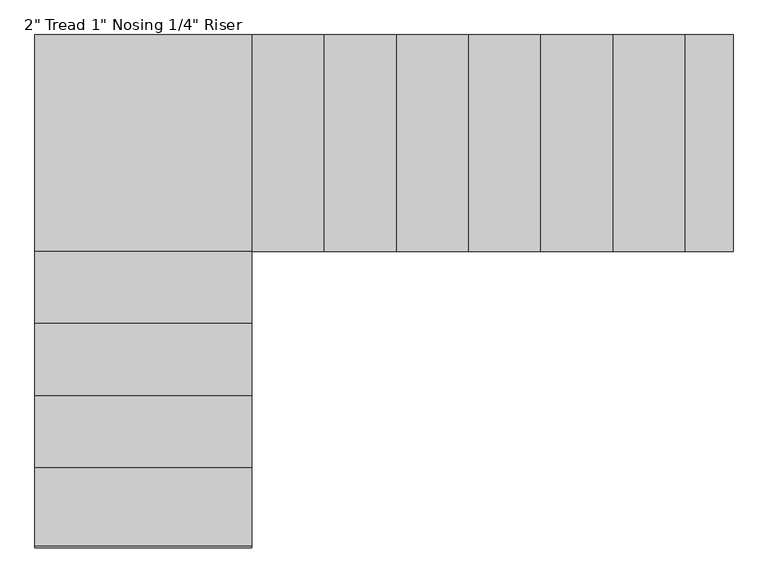
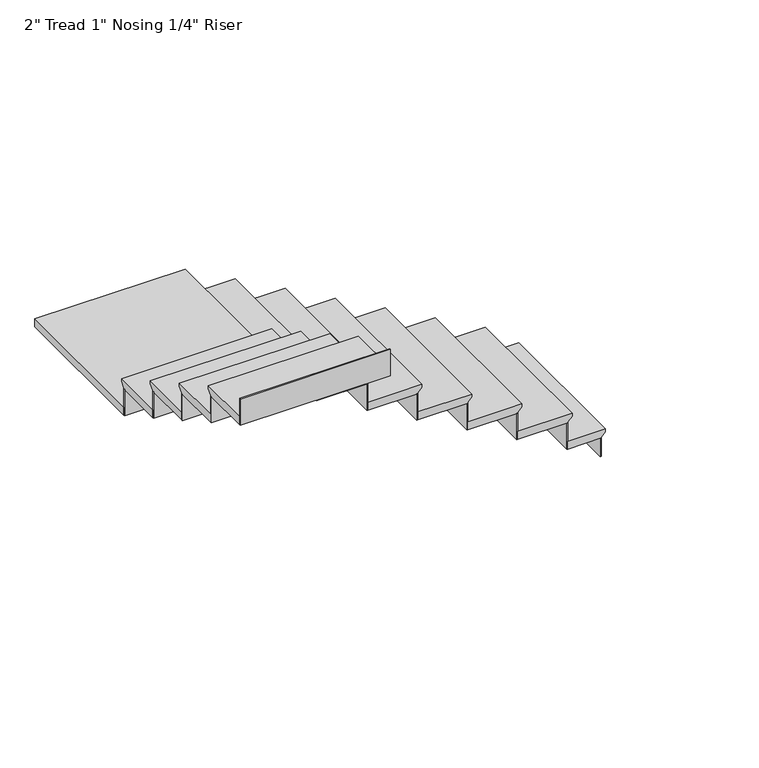
"""IFC4 building model written with IfcOpenShell, lengths in millimetres: stair flight geometry."""

from ifc_helpers import new_model, si_unit, origin, place, context, project, spatial, faceted_brep, source, transform, mapped, element, save


def stair_flight_aa7d7887(model_context):
    return source(origin(), model_context, "Body", "Brep", [
        faceted_brep([(-442.4415084, 5282.3381995, 9599.0833333), (-442.4415084, 5282.3381995, 9618.1333333), (-442.4415084, 4368.3146777, 9618.1333333), (-442.4415084, 4368.3146777, 9599.0833333), (-467.8415084, 5282.3381995, 9573.6833333), (-467.8415084, 4368.3146777, 9573.6833333), (-671.0415084, 5282.3381995, 9618.1333333), (-671.0415084, 4368.3146777, 9618.1333333), (-467.8415084, 4368.3146777, 9567.3333333), (-671.0415084, 4368.3146777, 9567.3333333), (-671.0415084, 5282.3381995, 9567.3333333), (-467.8415084, 5282.3381995, 9567.3333333)], [[[0, 1, 2, 3]], [[4, 0, 3, 5]], [[2, 1, 6, 7]], [[8, 9, 10, 11]], [[2, 7, 9, 8, 5, 3]], [[8, 11, 4, 5]], [[6, 1, 0, 4, 11, 10]], [[7, 6, 10, 9]]]),
        faceted_brep([(-467.8415084, 5282.3381995, 9567.3333333), (-467.8415084, 5282.3381995, 9448.8), (-474.1915084, 5282.3381995, 9448.8), (-474.1915084, 5282.3381995, 9567.3333333), (-467.8415084, 4368.3146777, 9567.3333333), (-474.1915084, 4368.3146777, 9567.3333333), (-474.1915084, 4368.3146777, 9448.8), (-467.8415084, 4368.3146777, 9448.8)], [[[0, 1, 2, 3]], [[4, 5, 6, 7]], [[1, 0, 4, 7]], [[2, 1, 7, 6]], [[3, 2, 6, 5]], [[0, 3, 5, 4]]]),
        faceted_brep([(-671.0415084, 5282.3381995, 9736.6666667), (-671.0415084, 5282.3381995, 9567.3333333), (-677.3915084, 5282.3381995, 9567.3333333), (-677.3915084, 5282.3381995, 9736.6666667), (-671.0415084, 4368.3146777, 9736.6666667), (-677.3915084, 4368.3146777, 9736.6666667), (-677.3915084, 4368.3146777, 9567.3333333), (-671.0415084, 4368.3146777, 9567.3333333)], [[[0, 1, 2, 3]], [[4, 5, 6, 7]], [[1, 0, 4, 7]], [[2, 1, 7, 6]], [[3, 2, 6, 5]], [[0, 3, 5, 4]]]),
        faceted_brep([(-645.6415084, 4368.3146777, 9787.4666667), (-645.6415084, 5282.3381995, 9787.4666667), (-975.8415084, 5282.3381995, 9787.4666667), (-975.8415084, 4368.3146777, 9787.4666667), (-671.0415084, 4368.3146777, 9736.6666667), (-975.8415084, 4368.3146777, 9736.6666667), (-975.8415084, 5282.3381995, 9736.6666667), (-671.0415084, 5282.3381995, 9736.6666667), (-671.0415084, 4368.3146777, 9743.0166667), (-645.6415084, 4368.3146777, 9768.4166667), (-671.0415084, 5282.3381995, 9743.0166667), (-645.6415084, 5282.3381995, 9768.4166667)], [[[0, 1, 2, 3]], [[4, 5, 6, 7]], [[0, 3, 5, 4, 8, 9]], [[4, 7, 10, 8]], [[2, 1, 11, 10, 7, 6]], [[3, 2, 6, 5]], [[11, 1, 0, 9]], [[10, 11, 9, 8]]]),
        faceted_brep([(-975.8415084, 5282.3381995, 9906.0), (-975.8415084, 5282.3381995, 9736.6666667), (-982.1915084, 5282.3381995, 9736.6666667), (-982.1915084, 5282.3381995, 9906.0), (-975.8415084, 4368.3146777, 9906.0), (-982.1915084, 4368.3146777, 9906.0), (-982.1915084, 4368.3146777, 9736.6666667), (-975.8415084, 4368.3146777, 9736.6666667)], [[[0, 1, 2, 3]], [[4, 5, 6, 7]], [[1, 0, 4, 7]], [[2, 1, 7, 6]], [[3, 2, 6, 5]], [[0, 3, 5, 4]]]),
        faceted_brep([(-950.4415084, 4368.3146777, 9956.8), (-950.4415084, 5282.3381995, 9956.8), (-1280.6415084, 5282.3381995, 9956.8), (-1280.6415084, 4368.3146777, 9956.8), (-975.8415084, 4368.3146777, 9906.0), (-1280.6415084, 4368.3146777, 9906.0), (-1280.6415084, 5282.3381995, 9906.0), (-975.8415084, 5282.3381995, 9906.0), (-975.8415084, 4368.3146777, 9912.35), (-950.4415084, 4368.3146777, 9937.75), (-975.8415084, 5282.3381995, 9912.35), (-950.4415084, 5282.3381995, 9937.75)], [[[0, 1, 2, 3]], [[4, 5, 6, 7]], [[0, 3, 5, 4, 8, 9]], [[4, 7, 10, 8]], [[2, 1, 11, 10, 7, 6]], [[3, 2, 6, 5]], [[11, 1, 0, 9]], [[10, 11, 9, 8]]]),
        faceted_brep([(-1280.6415084, 5282.3381995, 10075.3333333), (-1280.6415084, 5282.3381995, 9906.0), (-1286.9915084, 5282.3381995, 9906.0), (-1286.9915084, 5282.3381995, 10075.3333333), (-1280.6415084, 4368.3146777, 10075.3333333), (-1286.9915084, 4368.3146777, 10075.3333333), (-1286.9915084, 4368.3146777, 9906.0), (-1280.6415084, 4368.3146777, 9906.0)], [[[0, 1, 2, 3]], [[4, 5, 6, 7]], [[1, 0, 4, 7]], [[2, 1, 7, 6]], [[3, 2, 6, 5]], [[0, 3, 5, 4]]]),
        faceted_brep([(-1255.2415084, 4368.3146777, 10126.1333333), (-1255.2415084, 5282.3381995, 10126.1333333), (-1585.4415084, 5282.3381995, 10126.1333333), (-1585.4415084, 4368.3146777, 10126.1333333), (-1280.6415084, 4368.3146777, 10075.3333333), (-1585.4415084, 4368.3146777, 10075.3333333), (-1585.4415084, 5282.3381995, 10075.3333333), (-1280.6415084, 5282.3381995, 10075.3333333), (-1280.6415084, 4368.3146777, 10081.6833333), (-1255.2415084, 4368.3146777, 10107.0833333), (-1280.6415084, 5282.3381995, 10081.6833333), (-1255.2415084, 5282.3381995, 10107.0833333)], [[[0, 1, 2, 3]], [[4, 5, 6, 7]], [[0, 3, 5, 4, 8, 9]], [[4, 7, 10, 8]], [[2, 1, 11, 10, 7, 6]], [[3, 2, 6, 5]], [[11, 1, 0, 9]], [[10, 11, 9, 8]]]),
        faceted_brep([(-1585.4415084, 5282.3381995, 10244.6666667), (-1585.4415084, 5282.3381995, 10075.3333333), (-1591.7915084, 5282.3381995, 10075.3333333), (-1591.7915084, 5282.3381995, 10244.6666667), (-1585.4415084, 4368.3146777, 10244.6666667), (-1591.7915084, 4368.3146777, 10244.6666667), (-1591.7915084, 4368.3146777, 10075.3333333), (-1585.4415084, 4368.3146777, 10075.3333333)], [[[0, 1, 2, 3]], [[4, 5, 6, 7]], [[1, 0, 4, 7]], [[2, 1, 7, 6]], [[3, 2, 6, 5]], [[0, 3, 5, 4]]]),
        faceted_brep([(-1560.0415084, 4368.3146777, 10295.4666667), (-1560.0415084, 5282.3381995, 10295.4666667), (-1890.2415084, 5282.3381995, 10295.4666667), (-1890.2415084, 4368.3146777, 10295.4666667), (-1585.4415084, 4368.3146777, 10244.6666667), (-1890.2415084, 4368.3146777, 10244.6666667), (-1890.2415084, 5282.3381995, 10244.6666667), (-1585.4415084, 5282.3381995, 10244.6666667), (-1585.4415084, 4368.3146777, 10251.0166667), (-1560.0415084, 4368.3146777, 10276.4166667), (-1585.4415084, 5282.3381995, 10251.0166667), (-1560.0415084, 5282.3381995, 10276.4166667)], [[[0, 1, 2, 3]], [[4, 5, 6, 7]], [[0, 3, 5, 4, 8, 9]], [[4, 7, 10, 8]], [[2, 1, 11, 10, 7, 6]], [[3, 2, 6, 5]], [[11, 1, 0, 9]], [[10, 11, 9, 8]]]),
        faceted_brep([(-1890.2415084, 5282.3381995, 10414.0), (-1890.2415084, 5282.3381995, 10244.6666667), (-1896.5915084, 5282.3381995, 10244.6666667), (-1896.5915084, 5282.3381995, 10414.0), (-1890.2415084, 4368.3146777, 10414.0), (-1896.5915084, 4368.3146777, 10414.0), (-1896.5915084, 4368.3146777, 10244.6666667), (-1890.2415084, 4368.3146777, 10244.6666667)], [[[0, 1, 2, 3]], [[4, 5, 6, 7]], [[1, 0, 4, 7]], [[2, 1, 7, 6]], [[3, 2, 6, 5]], [[0, 3, 5, 4]]]),
        faceted_brep([(-1864.8415084, 4368.3146777, 10464.8), (-1864.8415084, 5282.3381995, 10464.8), (-2195.0415084, 5282.3381995, 10464.8), (-2195.0415084, 4368.3146777, 10464.8), (-1890.2415084, 4368.3146777, 10414.0), (-2195.0415084, 4368.3146777, 10414.0), (-2195.0415084, 5282.3381995, 10414.0), (-1890.2415084, 5282.3381995, 10414.0), (-1890.2415084, 4368.3146777, 10420.35), (-1864.8415084, 4368.3146777, 10445.75), (-1890.2415084, 5282.3381995, 10420.35), (-1864.8415084, 5282.3381995, 10445.75)], [[[0, 1, 2, 3]], [[4, 5, 6, 7]], [[0, 3, 5, 4, 8, 9]], [[4, 7, 10, 8]], [[2, 1, 11, 10, 7, 6]], [[3, 2, 6, 5]], [[11, 1, 0, 9]], [[10, 11, 9, 8]]]),
        faceted_brep([(-2195.0415084, 5282.3381995, 10583.3333333), (-2195.0415084, 5282.3381995, 10414.0), (-2201.3915084, 5282.3381995, 10414.0), (-2201.3915084, 5282.3381995, 10583.3333333), (-2195.0415084, 4368.3146777, 10583.3333333), (-2201.3915084, 4368.3146777, 10583.3333333), (-2201.3915084, 4368.3146777, 10414.0), (-2195.0415084, 4368.3146777, 10414.0)], [[[0, 1, 2, 3]], [[4, 5, 6, 7]], [[1, 0, 4, 7]], [[2, 1, 7, 6]], [[3, 2, 6, 5]], [[0, 3, 5, 4]]]),
        faceted_brep([(-2169.6415084, 4368.3146777, 10634.1333333), (-2169.6415084, 5282.3381995, 10634.1333333), (-2499.8415084, 5282.3381995, 10634.1333333), (-2499.8415084, 4368.3146777, 10634.1333333), (-2195.0415084, 4368.3146777, 10583.3333333), (-2499.8415084, 4368.3146777, 10583.3333333), (-2499.8415084, 5282.3381995, 10583.3333333), (-2195.0415084, 5282.3381995, 10583.3333333), (-2195.0415084, 4368.3146777, 10589.6833333), (-2169.6415084, 4368.3146777, 10615.0833333), (-2195.0415084, 5282.3381995, 10589.6833333), (-2169.6415084, 5282.3381995, 10615.0833333)], [[[0, 1, 2, 3]], [[4, 5, 6, 7]], [[0, 3, 5, 4, 8, 9]], [[4, 7, 10, 8]], [[2, 1, 11, 10, 7, 6]], [[3, 2, 6, 5]], [[11, 1, 0, 9]], [[10, 11, 9, 8]]]),
        faceted_brep([(-2499.8415084, 5282.3381995, 10752.6666667), (-2499.8415084, 5282.3381995, 10583.3333333), (-2506.1915084, 5282.3381995, 10583.3333333), (-2506.1915084, 5282.3381995, 10752.6666667), (-2499.8415084, 4368.3146777, 10752.6666667), (-2506.1915084, 4368.3146777, 10752.6666667), (-2506.1915084, 4368.3146777, 10583.3333333), (-2499.8415084, 4368.3146777, 10583.3333333)], [[[0, 1, 2, 3]], [[4, 5, 6, 7]], [[1, 0, 4, 7]], [[2, 1, 7, 6]], [[3, 2, 6, 5]], [[0, 3, 5, 4]]]),
        faceted_brep([(-3388.8415084, 5282.3381995, 10803.4666667), (-3388.8415084, 4342.9146777, 10803.4666667), (-2474.4415084, 4342.9146777, 10803.4666667), (-2474.4415084, 5282.3381995, 10803.4666667), (-2474.4415084, 4368.3146777, 10752.6666667), (-2474.4415084, 4342.9146777, 10752.6666667), (-3388.8415084, 4342.9146777, 10752.6666667), (-3388.8415084, 5282.3381995, 10752.6666667), (-2499.8415084, 5282.3381995, 10752.6666667), (-2499.8415084, 4368.3146777, 10752.6666667), (-2474.4415084, 4368.3146777, 10784.4166667), (-2474.4415084, 5282.3381995, 10784.4166667), (-2499.8415084, 4368.3146777, 10759.0166667), (-2499.8415084, 5282.3381995, 10759.0166667)], [[[0, 1, 2, 3]], [[4, 5, 6, 7, 8, 9]], [[3, 2, 5, 4, 10, 11]], [[4, 9, 12, 10]], [[9, 8, 13, 12]], [[0, 3, 11, 13, 8, 7]], [[1, 0, 7, 6]], [[2, 1, 6, 5]], [[13, 11, 10, 12]]]),
        faceted_brep([(-3388.8415084, 4342.9146777, 10922.0), (-3388.8415084, 4342.9146777, 10752.6666667), (-3388.8415084, 4336.5646777, 10752.6666667), (-3388.8415084, 4336.5646777, 10922.0), (-2474.4415084, 4342.9146777, 10922.0), (-2474.4415084, 4336.5646777, 10922.0), (-2474.4415084, 4336.5646777, 10752.6666667), (-2474.4415084, 4342.9146777, 10752.6666667)], [[[0, 1, 2, 3]], [[4, 5, 6, 7]], [[1, 0, 4, 7]], [[2, 1, 7, 6]], [[3, 2, 6, 5]], [[0, 3, 5, 4]]]),
        faceted_brep([(-2474.4415084, 4368.3146777, 10972.8), (-3388.8415084, 4368.3146777, 10972.8), (-3388.8415084, 4037.7382512, 10972.8), (-2474.4415084, 4037.7382512, 10972.8), (-2474.4415084, 4342.9146777, 10922.0), (-2474.4415084, 4037.7382512, 10922.0), (-3388.8415084, 4037.7382512, 10922.0), (-3388.8415084, 4342.9146777, 10922.0), (-2474.4415084, 4342.9146777, 10928.35), (-2474.4415084, 4368.3146777, 10953.75), (-3388.8415084, 4342.9146777, 10928.35), (-3388.8415084, 4368.3146777, 10953.75)], [[[0, 1, 2, 3]], [[4, 5, 6, 7]], [[0, 3, 5, 4, 8, 9]], [[4, 7, 10, 8]], [[2, 1, 11, 10, 7, 6]], [[3, 2, 6, 5]], [[11, 1, 0, 9]], [[10, 11, 9, 8]]]),
        faceted_brep([(-3388.8415084, 4037.7382512, 11091.3333333), (-3388.8415084, 4037.7382512, 10922.0), (-3388.8415084, 4031.3882512, 10922.0), (-3388.8415084, 4031.3882512, 11091.3333333), (-2474.4415084, 4037.7382512, 11091.3333333), (-2474.4415084, 4031.3882512, 11091.3333333), (-2474.4415084, 4031.3882512, 10922.0), (-2474.4415084, 4037.7382512, 10922.0)], [[[0, 1, 2, 3]], [[4, 5, 6, 7]], [[1, 0, 4, 7]], [[2, 1, 7, 6]], [[3, 2, 6, 5]], [[0, 3, 5, 4]]]),
        faceted_brep([(-2474.4415084, 4063.1382512, 11142.1333333), (-3388.8415084, 4063.1382512, 11142.1333333), (-3388.8415084, 3732.938277, 11142.1333333), (-2474.4415084, 3732.938277, 11142.1333333), (-2474.4415084, 4037.7382512, 11091.3333333), (-2474.4415084, 3732.938277, 11091.3333333), (-3388.8415084, 3732.938277, 11091.3333333), (-3388.8415084, 4037.7382512, 11091.3333333), (-2474.4415084, 4037.7382512, 11097.6833333), (-2474.4415084, 4063.1382512, 11123.0833333), (-3388.8415084, 4037.7382512, 11097.6833333), (-3388.8415084, 4063.1382512, 11123.0833333)], [[[0, 1, 2, 3]], [[4, 5, 6, 7]], [[0, 3, 5, 4, 8, 9]], [[4, 7, 10, 8]], [[2, 1, 11, 10, 7, 6]], [[3, 2, 6, 5]], [[11, 1, 0, 9]], [[10, 11, 9, 8]]]),
        faceted_brep([(-3388.8415084, 3732.938277, 11260.6666667), (-3388.8415084, 3732.938277, 11091.3333333), (-3388.8415084, 3726.588277, 11091.3333333), (-3388.8415084, 3726.588277, 11260.6666667), (-2474.4415084, 3732.938277, 11260.6666667), (-2474.4415084, 3726.588277, 11260.6666667), (-2474.4415084, 3726.588277, 11091.3333333), (-2474.4415084, 3732.938277, 11091.3333333)], [[[0, 1, 2, 3]], [[4, 5, 6, 7]], [[1, 0, 4, 7]], [[2, 1, 7, 6]], [[3, 2, 6, 5]], [[0, 3, 5, 4]]]),
        faceted_brep([(-2474.4415084, 3758.338277, 11311.4666667), (-3388.8415084, 3758.338277, 11311.4666667), (-3388.8415084, 3428.1383028, 11311.4666667), (-2474.4415084, 3428.1383028, 11311.4666667), (-2474.4415084, 3732.938277, 11260.6666667), (-2474.4415084, 3428.1383028, 11260.6666667), (-3388.8415084, 3428.1383028, 11260.6666667), (-3388.8415084, 3732.938277, 11260.6666667), (-2474.4415084, 3732.938277, 11267.0166667), (-2474.4415084, 3758.338277, 11292.4166667), (-3388.8415084, 3732.938277, 11267.0166667), (-3388.8415084, 3758.338277, 11292.4166667)], [[[0, 1, 2, 3]], [[4, 5, 6, 7]], [[0, 3, 5, 4, 8, 9]], [[4, 7, 10, 8]], [[2, 1, 11, 10, 7, 6]], [[3, 2, 6, 5]], [[11, 1, 0, 9]], [[10, 11, 9, 8]]]),
        faceted_brep([(-3388.8415084, 3428.1383028, 11430.0), (-3388.8415084, 3428.1383028, 11260.6666667), (-3388.8415084, 3421.7883028, 11260.6666667), (-3388.8415084, 3421.7883028, 11430.0), (-2474.4415084, 3428.1383028, 11430.0), (-2474.4415084, 3421.7883028, 11430.0), (-2474.4415084, 3421.7883028, 11260.6666667), (-2474.4415084, 3428.1383028, 11260.6666667)], [[[0, 1, 2, 3]], [[4, 5, 6, 7]], [[1, 0, 4, 7]], [[2, 1, 7, 6]], [[3, 2, 6, 5]], [[0, 3, 5, 4]]]),
        faceted_brep([(-3388.8415084, 3123.3383287, 11599.3333333), (-3388.8415084, 3123.3383287, 11430.0), (-3388.8415084, 3116.9883287, 11430.0), (-3388.8415084, 3116.9883287, 11599.3333333), (-2474.4415084, 3123.3383287, 11599.3333333), (-2474.4415084, 3116.9883287, 11599.3333333), (-2474.4415084, 3116.9883287, 11430.0), (-2474.4415084, 3123.3383287, 11430.0)], [[[0, 1, 2, 3]], [[4, 5, 6, 7]], [[1, 0, 4, 7]], [[2, 1, 7, 6]], [[3, 2, 6, 5]], [[0, 3, 5, 4]]]),
        faceted_brep([(-2474.4415084, 3453.5383028, 11480.8), (-3388.8415084, 3453.5383028, 11480.8), (-3388.8415084, 3123.3383287, 11480.8), (-2474.4415084, 3123.3383287, 11480.8), (-2474.4415084, 3428.1383028, 11430.0), (-2474.4415084, 3123.3383287, 11430.0), (-3388.8415084, 3123.3383287, 11430.0), (-3388.8415084, 3428.1383028, 11430.0), (-2474.4415084, 3428.1383028, 11436.35), (-2474.4415084, 3453.5383028, 11461.75), (-3388.8415084, 3428.1383028, 11436.35), (-3388.8415084, 3453.5383028, 11461.75)], [[[0, 1, 2, 3]], [[4, 5, 6, 7]], [[0, 3, 5, 4, 8, 9]], [[4, 7, 10, 8]], [[2, 1, 11, 10, 7, 6]], [[3, 2, 6, 5]], [[11, 1, 0, 9]], [[10, 11, 9, 8]]]),
    ])


if __name__ == "__main__":
    model = new_model("IFC4")
    model_context = context("Model", 3, world=origin())
    ifc_project = project(units=[si_unit("LENGTHUNIT", "METRE", prefix="MILLI")], contexts=[model_context])
    site = spatial("IfcSite", under=ifc_project)
    building = spatial("IfcBuilding", under=site)
    placement = place(None, origin())
    stair_flight_shape = stair_flight_aa7d7887(model_context)
    element("IfcStairFlight", 1, ObjectType="2\" Tread 1\" Nosing 1/4\" Riser", at=placement, inside=building, context=model_context, shape_type="MappedRepresentation", body=[
        mapped(stair_flight_shape, transform((0.0, 0.0, 0.0), x_axis=(1.0, 0.0, 0.0), y_axis=(0.0, 1.0, 0.0), z_axis=(0.0, 0.0, 1.0))),
    ])
    save(model, "model.ifc")
